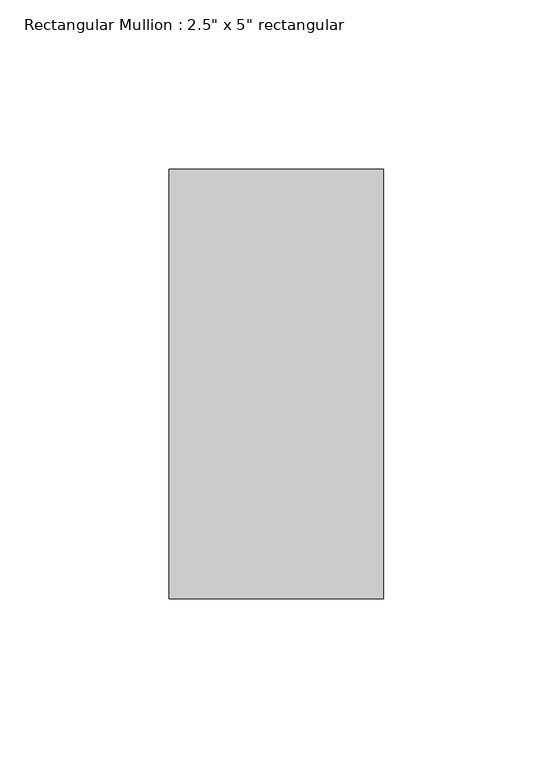
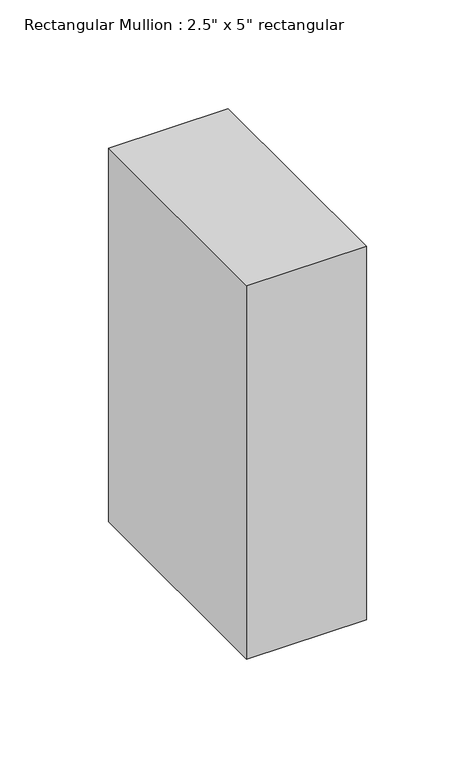
"""IFC4 building model written with IfcOpenShell, lengths in millimetres: member geometry."""

from ifc_helpers import new_model, si_unit, frame, origin, place, context, project, spatial, polyline, outline, extrude, source, transform, mapped, element, save


def member_a5966c2a(model_context):
    return source(origin(), model_context, "Body", "SweptSolid", [
        extrude(outline(polyline([(31.75, 63.5), (31.75, -63.5), (-31.75, -63.5), (-31.75, 63.5), (31.75, 63.5)])), frame((0.0, 0.0, -209.55), z_axis=(0.0, 0.0, 1.0), x_axis=(1.0, 0.0, 0.0)), (0.0, 0.0, 1.0), 209.55),
    ])


if __name__ == "__main__":
    model = new_model("IFC4")
    model_context = context("Model", 3, world=origin())
    ifc_project = project(units=[si_unit("LENGTHUNIT", "METRE", prefix="MILLI")], contexts=[model_context])
    site = spatial("IfcSite", under=ifc_project)
    building = spatial("IfcBuilding", under=site)
    placement = place(None, origin())
    member_shape = member_a5966c2a(model_context)
    element("IfcMember", 1, ObjectType="Rectangular Mullion : 2.5\" x 5\" rectangular", at=placement, inside=building, context=model_context, shape_type="MappedRepresentation", body=[
        mapped(member_shape, transform((0.0, 0.0, 0.0), x_axis=(1.0, 0.0, 0.0), y_axis=(0.0, 1.0, 0.0), z_axis=(0.0, 0.0, 1.0))),
    ])
    save(model, "model.ifc")

# Revit data of these elements
# Type "Rectangular Mullion : 2.5\" x 5\" rectangular"
#   built-in parameter 1007304 = 0.416667 (stored number, unit not read)
#   built-in parameter 1007301 = 0.104167 (stored number, unit not read)
#   built-in parameter 1007300 = 0.104167 (stored number, unit not read)
# Element 1 (IfcMember, "Rectangular Mullion : 2.5\" x 5\" rectangular")
#   Materials on its faces: "Aluminum"
# Materials
#   "Aluminum": class "Metal", colour RGB 247 247 247, transparency 0, Description = "Aluminum 6061", Cost = 0
